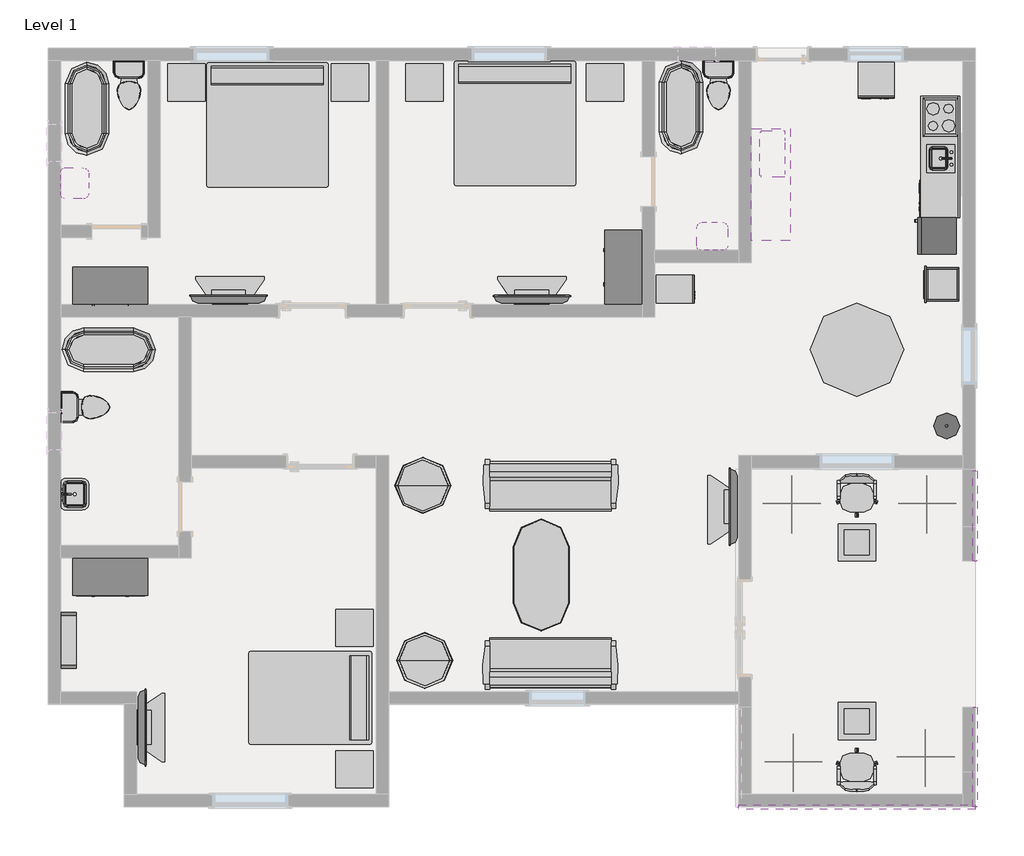
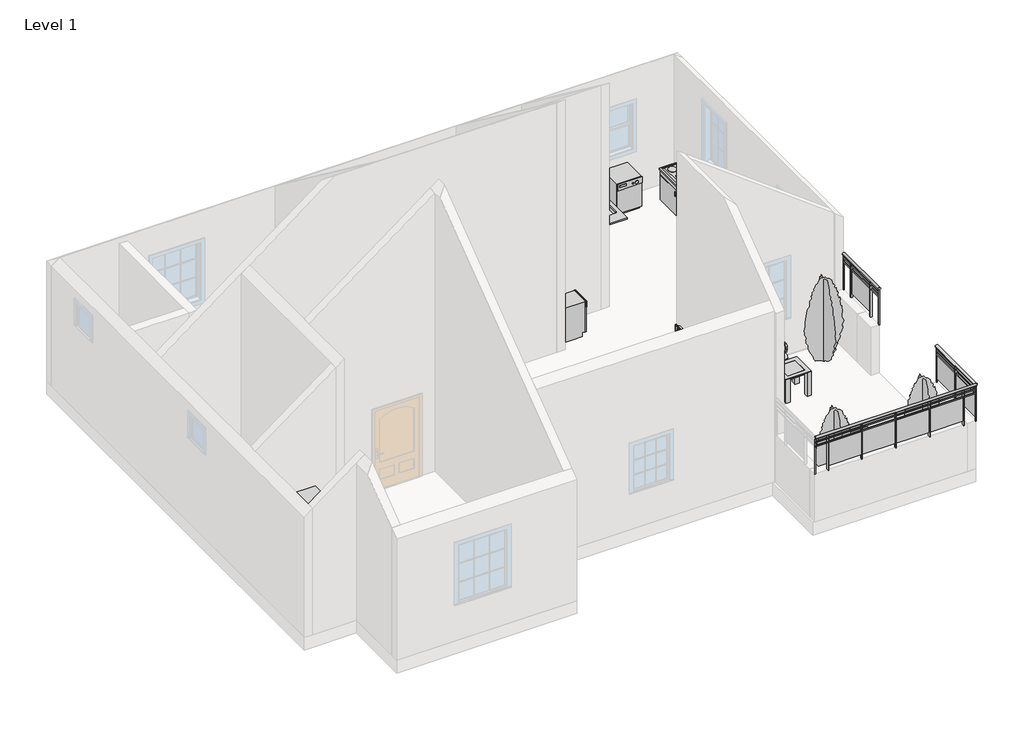
# One storey, part 2 of 2: 33 furniture elements, 11 flow terminals, 8 proxies, 4 geographic elements, 3 railings.
# Revit data of these elements (continued)
# Materials (continued)
#   "Laminate, Linen, Matte": class "Plastic", colour RGB 249 239 230, transparency 0, Description = "Plastic Laminate - Linen, Matte", Cost = 0
#   "Porcelain, Ivory": class "Ceramic", colour RGB 247 247 239, transparency 0, Description = "Porcelain, ivory", Cost = 0
#   "Linen, White": class "Textile", colour RGB 247 247 239, transparency 0, Description = "Linen, white", Cost = 0
#   "Textile - Slate Blue": class "Fabric", colour RGB 98 102 118, transparency 0
#   "Laminate - Ivory, Glossy": colour RGB 247 247 239, transparency 0
#   "Cherry": class "Wood", colour RGB 226 177 128, transparency 0, Description = "Prunus Serotina", Cost = 0
#   "Birch": class "Wood", colour RGB 224 178 126, transparency 0, Description = "Betula Alleghaniensis", Cost = 0
#   "Linen, Beige": class "Textile", colour RGB 249 239 230, transparency 0, Description = "Linen, beige", Cost = 0
#   "Melamine - Gray": class "Wood", colour RGB 49 49 49, transparency 0
#   "Glass - Clear, Grey": class "Glass", colour RGB 252 255 255, transparency 0.64
#   "Pine": class "Wood", colour RGB 223 192 134, transparency 0, Description = "Pinus Echinata", Cost = 0
#   "Glass": class "Glass", colour RGB 0 128 192, transparency 0.75, Description = "Soda Lime Glass", Cost = 0
#   "Steel": class "Metal", colour RGB 247 247 247, transparency 0, Description = "Steel, mill finish", Cost = 0
#   "Counter Top": class "Wood", colour RGB 226 177 128, transparency 0
#   "TV - Black": colour RGB 49 49 49, transparency 0
#   "TV - Glass": colour RGB 157 157 157, transparency 0.9
#   "TV - Screen": colour RGB 0 0 0, transparency 0
#   "Glass - Shelves": class "Glass", colour RGB 167 167 167, transparency 0.9
